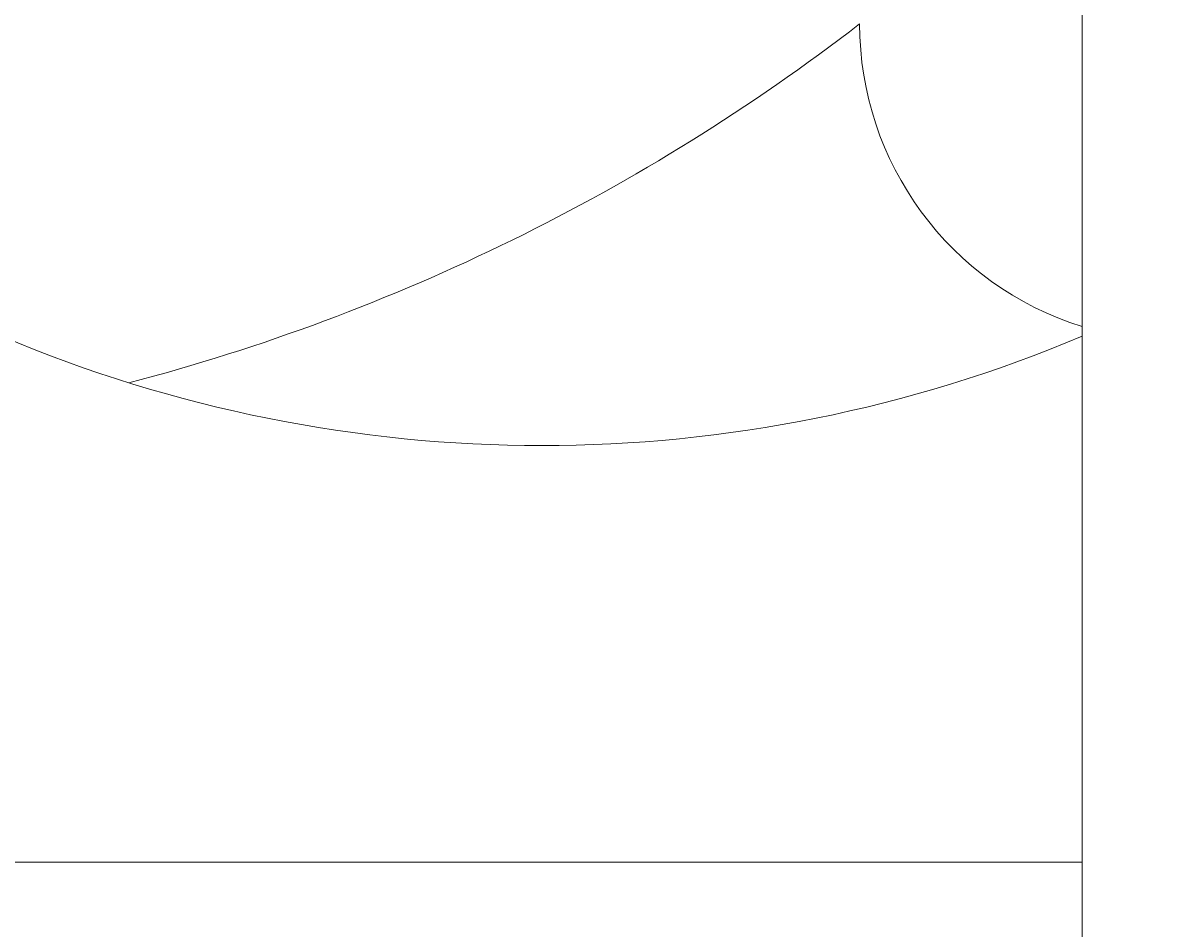
# Model space of a CAD drawing. Units: inches. Extents: x -46 to 1145, y -527 to 760.
# Tile 29 of 57: x 79 to 111, y 252 to 277. Entities that reach past the tile are written whole.
import ezdxf

# ---------------------------------------------------------------- set-up
doc = ezdxf.new("R2010")
doc.units = ezdxf.units.IN
doc.header["$MEASUREMENT"] = 0
doc.layers.add('A-ANNO-DIMS', color=2, linetype='Continuous', lineweight=18)
doc.layers.add('A-FURN', color=2, linetype='Continuous', lineweight=13)
doc.styles.get("Standard").update_dxf_attribs({"font": 'arial.ttf'})
doc.dimstyles.get("Standard").update_dxf_attribs({"dimtxt": 0.18, "dimasz": 0.18, "dimexe": 0.18, "dimexo": 0.0625, "dimgap": 0.09, "dimtad": 0, "dimtih": 1, "dimtoh": 1, "dimdec": 0, "dimzin": 0, "dimdsep": 46, "dimlunit": 3, "dimtxsty": 'Standard', "dimcen": 0.09, "dimadec": 0, "dimazin": 0, "dimtfac": 1, "dimtdec": 0, "dimtofl": 0, "dimtmove": 0, "dimatfit": 3, "dimfxl": 1, "dimtolj": 1, "dimtzin": 0, "dimarcsym": 0})

# ---------------------------------------------------------------- blocks, each defined once
blk = doc.blocks.new('BED-QUEEN-FURNISHED')
for p, q in [((0, 0), (0, 80)), ((60, 63.2), (0, 63.2))]:
    blk.add_line(p, q)
for centre, radius, start, end in [((15, 13.075), 38.562, 67.1089, 112.8911), ((40.884, -5.132), 56.884, 104.6834, 127.6009), ((-2.624, 39.936), 8.8, 0, 72.6522)]:
    blk.add_arc(centre, radius, start, end)
blk = doc.blocks.new('*D685')
at = {"layer": 'A-ANNO-DIMS', "color": 0, "lineweight": -2, "transparency": 16777216}
for p, q in [((183.501, 700.889), (-46.216, 700.889)), ((-46.036, 700.709), (-46.036, 116.385)), ((-46.036, -468.302), (-46.036, 116.021)), ((12.501, -468.482), (-46.216, -468.482))]:
    blk.add_line(p, q, dxfattribs=at)
at = {"layer": 'A-ANNO-DIMS', "color": 0, "transparency": 16777216}
for points in [[(-46.066, 700.709), (-46.006, 700.709), (-46.036, 700.889)], [(-46.066, -468.302), (-46.006, -468.302), (-46.036, -468.482)]]:
    blk.add_solid(points, dxfattribs=at)
at = {"layer": 'Defpoints', "color": 0, "transparency": 16777216}
for p in [(-46.036, 700.889), (183.564, 700.889), (12.564, -468.482)]:
    blk.add_point(p, dxfattribs=at)
at = {"layer": 'A-ANNO-DIMS', "color": 0, "transparency": 16777216, "insert": (-46.036, 116.203), "char_height": 0.18, "attachment_point": 5}
blk.add_mtext('\\A1;1169.4', dxfattribs=at)

msp = doc.modelspace()

# ---------------------------------------------------------------- block references
at = {"layer": 'A-FURN', "rotation": 180}
msp.add_blockref('BED-QUEEN-FURNISHED', (108.4877, 316.6818), dxfattribs=at)

# ---------------------------------------------------------------- dimensions: what is measured, and where the dimension line sits
at = {"layer": 'A-ANNO-DIMS'}
dim = msp.add_linear_dim(base=(-46.0363, 700.8886), p1=(12.5637, -468.4824), p2=(183.5637, 700.8886), angle=90, dimstyle='Standard', override={"dimdec": 1, "dimlfac": 1, "dimrnd": 0, "dimzin": 0, "dimdsep": 46, "dimlunit": 2}, dxfattribs=at)
dim.commit()
dim.dimension.update_dxf_attribs({"geometry": '*D685', "text_midpoint": (-46.0363, 116.2031)})

doc.saveas('drawing.dxf')
